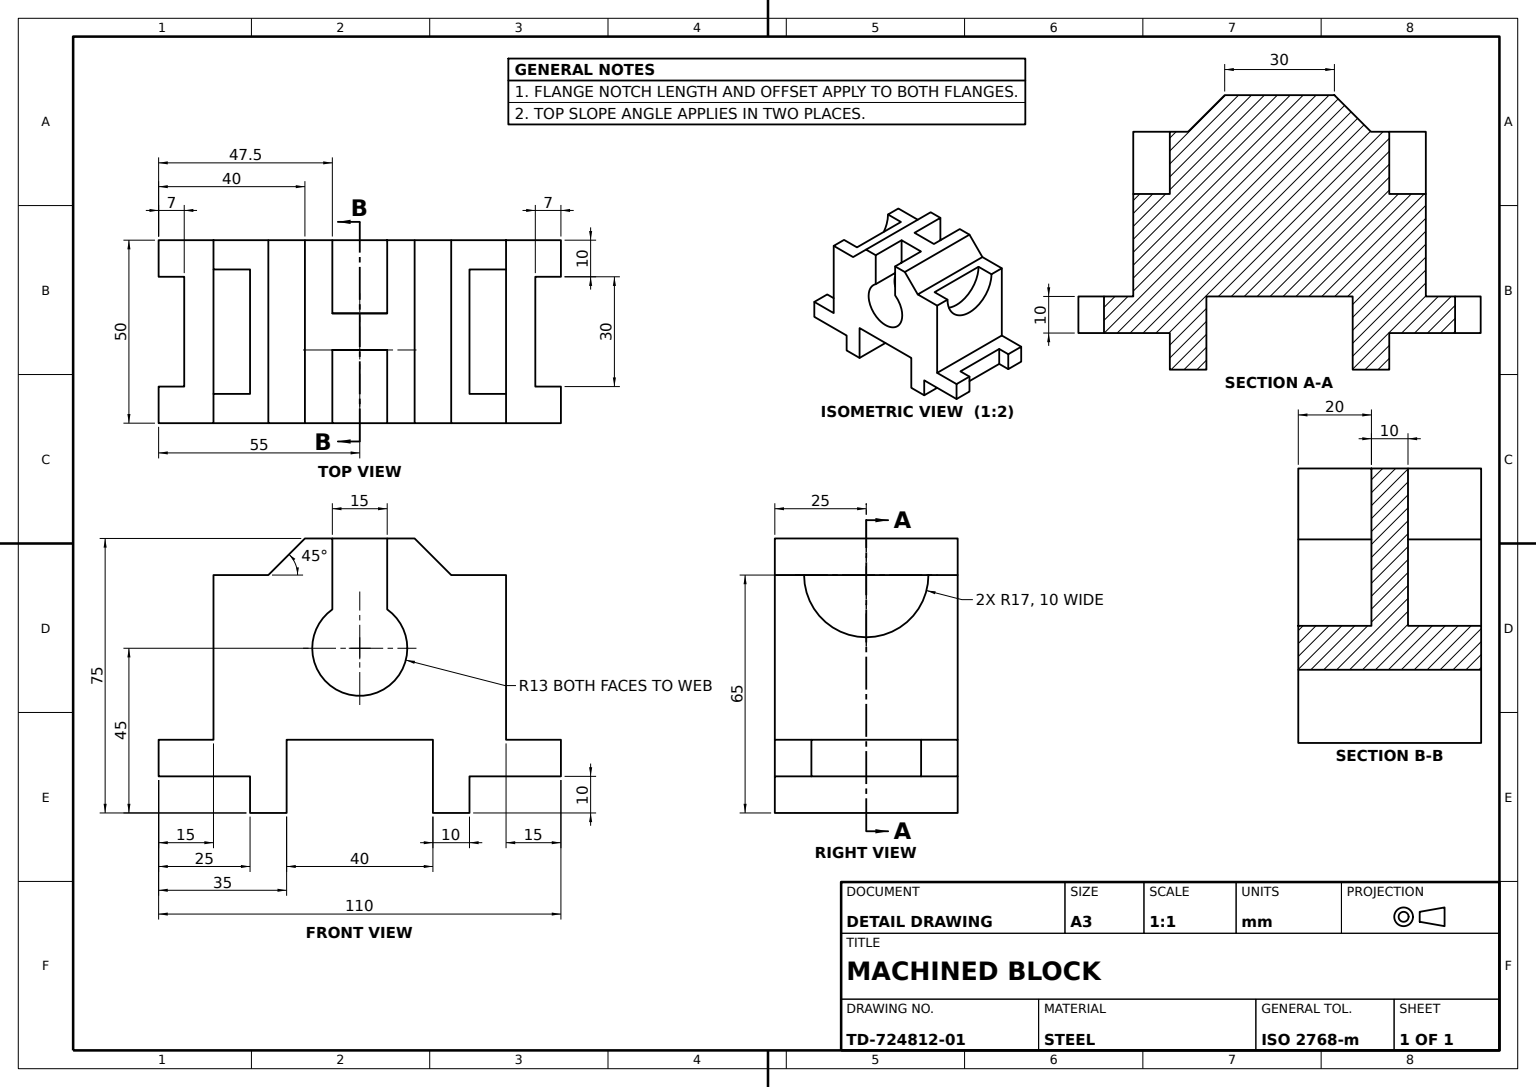
from build123d import *

# Parameters (mm, degrees)
BASE_BODY_DEPTH          = 50
UPPER_BLOCK_DEPTH        = 50
CENTRE_START             = -10
CENTRE_WEB_DEPTH         = 10
FOOT_SLOT_1_DEPTH        = 7
FOOT_SLOT_2_DEPTH        = 7
BEARING_SEAT_CUT_1_DEPTH = 10
BEARING_START            = -10
BEARING_SEAT_CUT_2_DEPTH = 10


with BuildPart() as part:
    # Base Body Profile Sketch → Base Body (new body)
    with BuildSketch(Plane.XY):
        with BuildLine():
            Line((0, 0), (25, 0))
            Line((25, 0), (25, -10))
            Line((25, -10), (35, -10))
            Line((35, -10), (35, 10))
            Line((35, 10), (75, 10))
            Line((75, 10), (75, -10))
            Line((75, -10), (85, -10))
            Line((85, -10), (85, 0))
            Line((85, 0), (110, 0))
            Line((110, 0), (110, 10))
            Line((110, 10), (95, 10))
            Line((95, 10), (95, 55))
            Line((95, 55), (80, 55))
            Line((80, 55), (70, 65))
            Line((70, 65), (62.5, 65))
            Line((62.5, 65), (62.5, 48))
            Line((62.5, 48), (62.5, 45.618380291))
            ThreePointArc((62.5, 45.618380291), (55, 22), (47.5, 45.618380291))
            Line((47.5, 45.618380291), (47.5, 48))
            Line((47.5, 48), (47.5, 65))
            Line((47.5, 65), (40, 65))
            Line((40, 65), (30, 55))
            Line((30, 55), (15, 55))
            Line((15, 55), (15, 10))
            Line((15, 10), (0, 10))
            Line((0, 10), (0, 0))
        make_face()
    extrude(amount=BASE_BODY_DEPTH)

    # Upper Block Sketch → Upper Block (add)
    with BuildSketch(Plane(origin=(0, 65, 0), x_dir=(1, 0, 0), z_dir=(0, 1, 0))):
        Polygon((47.5, -20), (47.5, -25), (47.5, -30), (62.5, -30), (62.5, -20), align=None)
    extrude(amount=-UPPER_BLOCK_DEPTH)

    # Centre Web Sketch → Centre Web (add)
    with BuildSketch(Plane.XY.offset(30).offset(CENTRE_START)):
        with BuildLine():
            Line((47.5, 45.618380291), (47.5, 24.381619709))
            ThreePointArc((47.5, 24.381619709), (42, 35), (47.5, 45.618380291))
        make_face()
        with BuildLine():
            Line((62.5, 45.618380291), (62.5, 24.381619709))
            ThreePointArc((62.5, 24.381619709), (68, 35), (62.5, 45.618380291))
        make_face()
    extrude(amount=CENTRE_WEB_DEPTH)

    # Foot Slot 1 Sketch → Foot Slot 1 (cut)
    with BuildSketch(Plane.ZY):
        Polygon((25, 10), (10, 10), (10, 0), (40, 0), (40, 10), align=None)
    extrude(amount=-FOOT_SLOT_1_DEPTH, mode=Mode.SUBTRACT)

    # Foot Slot 2 Sketch → Foot Slot 2 (cut)
    with BuildSketch(Plane(origin=(110, 0, 0), x_dir=(0, 0, -1), z_dir=(1, 0, 0))):
        Polygon((-25, 10), (-40, 10), (-40, 0), (-10, 0), (-10, 10), align=None)
    extrude(amount=-FOOT_SLOT_2_DEPTH, mode=Mode.SUBTRACT)

    # Bearing Seat Cut 1 Sketch → Bearing Seat Cut 1 (cut)
    with BuildSketch(Plane(origin=(95, 0, 0), x_dir=(0, 0, -1), z_dir=(1, 0, 0))):
        with BuildLine():
            Line((-42, 55), (-8, 55))
            ThreePointArc((-8, 55), (-25, 38), (-42, 55))
        make_face()
    extrude(amount=-BEARING_SEAT_CUT_1_DEPTH, mode=Mode.SUBTRACT)

    # Bearing Seat Cut 2 Sketch → Bearing Seat Cut 2 (cut)
    with BuildSketch(Plane.ZY.offset(-15).offset(BEARING_START)):
        with BuildLine():
            Line((8, 55), (42, 55))
            ThreePointArc((42, 55), (25, 38), (8, 55))
        make_face()
    extrude(amount=BEARING_SEAT_CUT_2_DEPTH, mode=Mode.SUBTRACT)


solid = part.part
